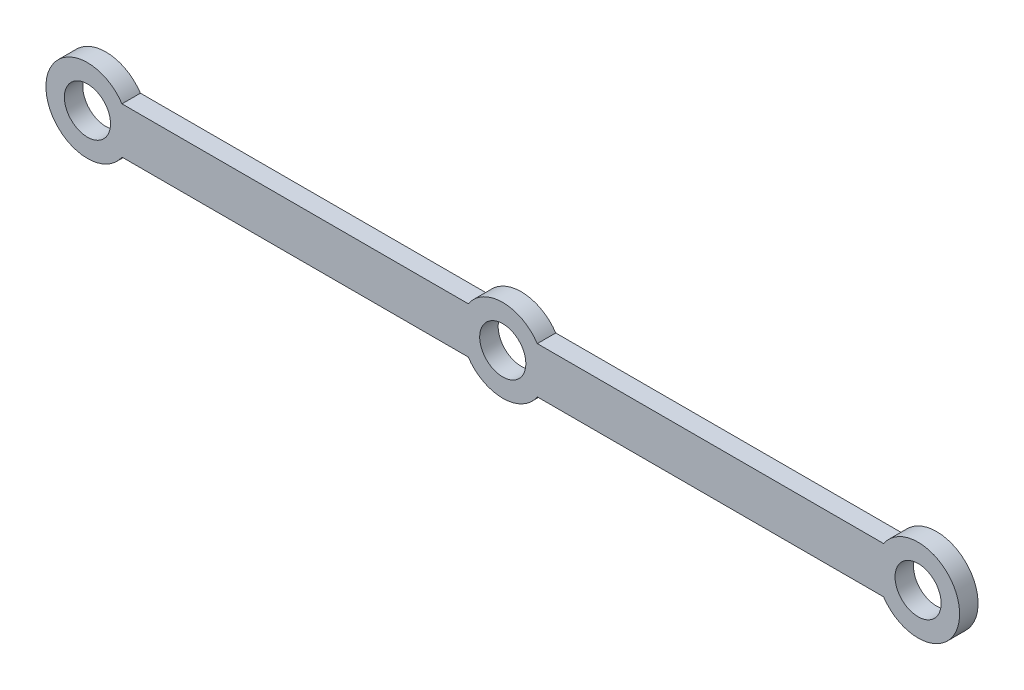
SolidWorks part; units mm, degrees
material "Plain Carbon Steel"
ref_plane "Front Plane" through (0, 0, 0) normal (0, 0, 1) x (1, 0, 0)
ref_plane "Top Plane" through (0, 0, 0) normal (0, 1, 0) x (1, 0, 0)
ref_plane "Right Plane" through (0, 0, 0) normal (1, 0, 0) x (0, 0, -1)
sketch "Link Profile Sketch" plane through (0, 0, 0) normal (0, 0, 1) x (1, 0, 0)
  line L0 (3.7417, 2.5) -> (41.2583, 2.5)
  line L5 (-45, 0) -> (45, 0) construction
  line L6 (3.7417, -2.5) -> (41.2583, -2.5)
  line L7 (-41.2583, 2.5) -> (-3.7417, 2.5)
  line L8 (-41.2583, -2.5) -> (-3.7417, -2.5)
  arc A0 (-41.2583, 2.5) -> (-41.2583, -2.5) centre (-45, 0) ccw
  arc A1 (-3.7417, -2.5) -> (3.7417, -2.5) centre (0, 0) ccw
  arc A2 (41.2583, -2.5) -> (41.2583, 2.5) centre (45, 0) ccw
  arc A3 (3.7417, 2.5) -> (-3.7417, 2.5) centre (0, 0) ccw
  circle A4 centre (-45, 0) radius 2.5
  circle A5 centre (0, 0) radius 2.5
  circle A6 centre (45, 0) radius 2.5
  dimension "D5" = 5
  dimension "D4" = 9
  dimension "D1" = 90
  dimension "D2" = 5
  dimension "D3" = 45
extrude "Link Plate 2mm" add sketch "Link Profile Sketch" along normal mid plane 2
